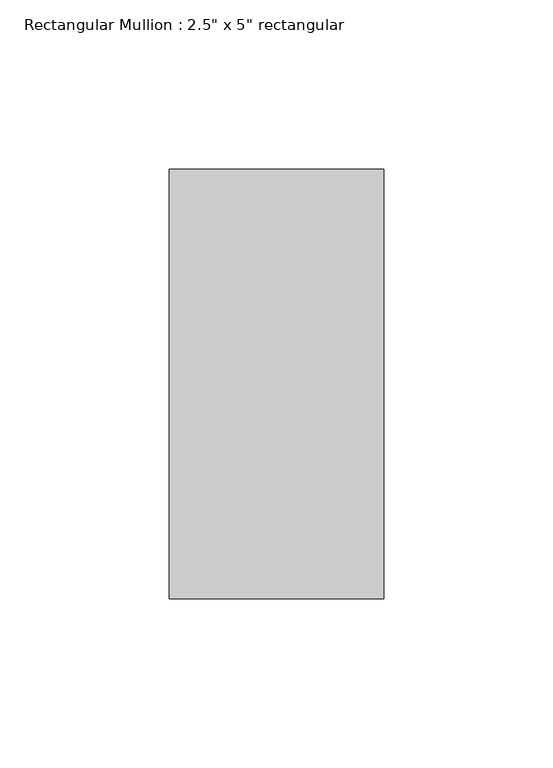
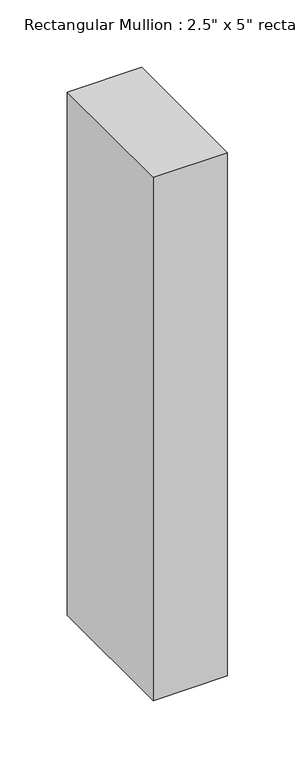
"""IFC4 building model written with IfcOpenShell, lengths in millimetres: member geometry."""

from ifc_helpers import new_model, si_unit, frame, origin, place, context, project, spatial, polyline, outline, extrude, source, transform, mapped, element, save


def member_f3b54ad7(model_context):
    return source(origin(), model_context, "Body", "SweptSolid", [
        extrude(outline(polyline([(0.0, 63.5), (0.0, -63.5), (-63.5, -63.5), (-63.5, 63.5), (0.0, 63.5)])), frame((0.0, 0.0, -473.2270844), z_axis=(0.0, 0.0, 1.0), x_axis=(1.0, 0.0, 0.0)), (0.0, 0.0, 1.0), 473.2270844),
    ])


if __name__ == "__main__":
    model = new_model("IFC4")
    model_context = context("Model", 3, world=origin())
    ifc_project = project(units=[si_unit("LENGTHUNIT", "METRE", prefix="MILLI")], contexts=[model_context])
    site = spatial("IfcSite", under=ifc_project)
    building = spatial("IfcBuilding", under=site)
    placement = place(None, origin())
    member_shape = member_f3b54ad7(model_context)
    element("IfcMember", 1, ObjectType="Rectangular Mullion : 2.5\" x 5\" rectangular", at=placement, inside=building, context=model_context, shape_type="MappedRepresentation", body=[
        mapped(member_shape, transform((0.0, 0.0, 0.0), x_axis=(1.0, 0.0, 0.0), y_axis=(0.0, 1.0, 0.0), z_axis=(0.0, 0.0, 1.0))),
    ])
    save(model, "model.ifc")

# Revit data of these elements
# Type "Rectangular Mullion : 2.5\" x 5\" rectangular"
#   built-in parameter 1007304 = 0.416667 (stored number, unit not read)
#   built-in parameter 1007301 = 0.104167 (stored number, unit not read)
#   built-in parameter 1007300 = 0.104167 (stored number, unit not read)
# Element 1 (IfcMember, "Rectangular Mullion : 2.5\" x 5\" rectangular")
#   Materials on its faces: "Aluminum"
# Materials
#   "Aluminum": class "Metal", colour RGB 247 247 247, transparency 0, Description = "Aluminum 6061", Cost = 0
